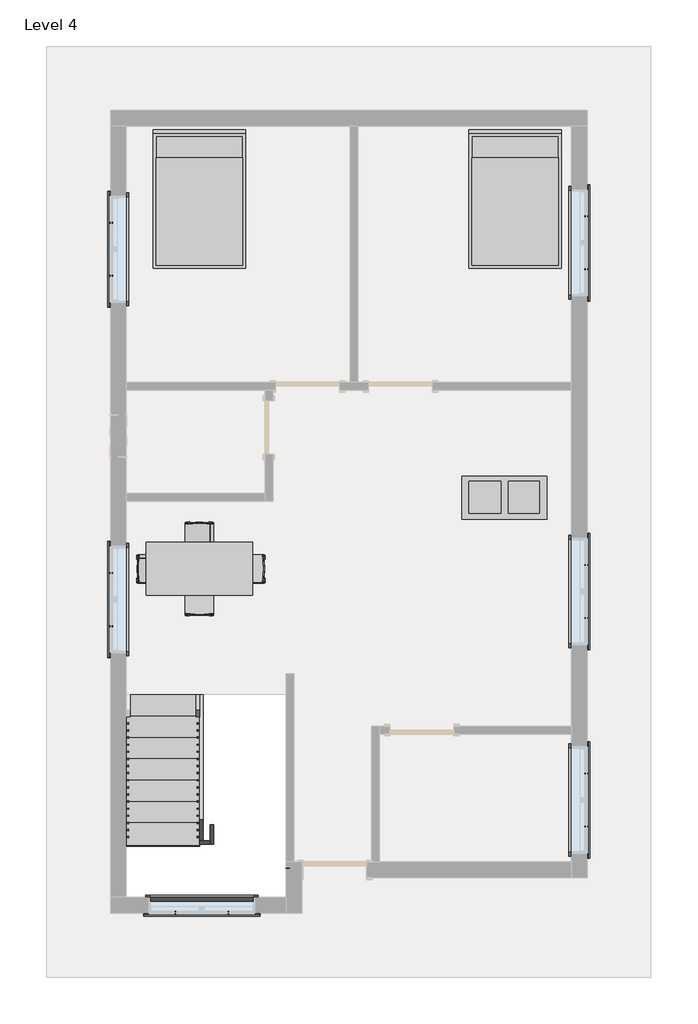
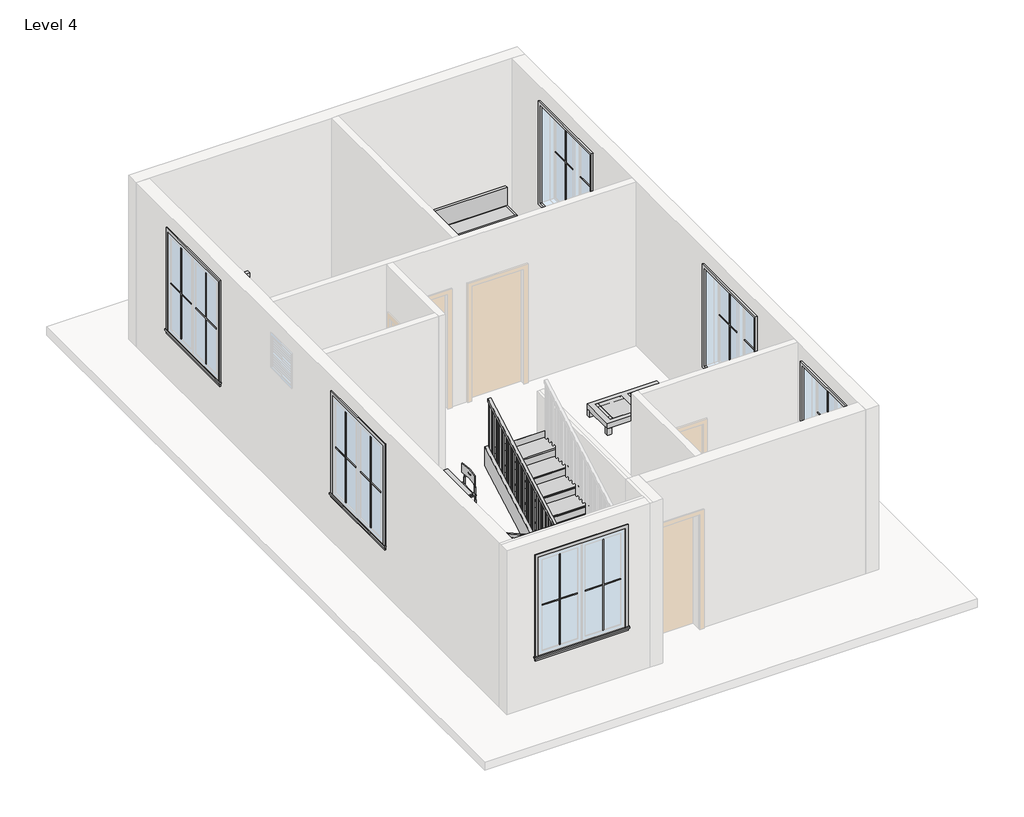
# One storey, part 3 of 3: 25 proxies, 6 members, 3 furniture elements, 1 railing, 1 stair flight.
"""IFC4 building model written with IfcOpenShell, lengths in millimetres."""

from ifc_helpers import new_model, si_unit, frame, origin, place, context, project, spatial, polyline, outline, extrude, faceted_brep, transform, mapped, element, save
from components import muntin_pattern_2x2_muntin_pattern_2x2_f6a80940, muntin_pattern_2x2_muntin_pattern_2x2_09b00a1c, trim_window_exterior_flat_with_sill_698ed857, trim_window_interior_flat_picture_frame_92551a5e, coffee_table_with_brass_mullions_11320_coffee_table_with_5962bef7, bed_17739_bed_17739_15c61121, dining_table_w_chairs_11374_0cdfc61b, stair_flight_f9143c42

model = new_model("IFC4")

# Units and contexts
model_context = context("Model", 3, world=origin())
ifc_project = project(units=[si_unit("LENGTHUNIT", "METRE", prefix="MILLI")], contexts=[model_context])

# Site, building, storey
site = spatial("IfcSite", under=ifc_project)
building = spatial("IfcBuilding", under=site)
storey = spatial("IfcBuildingStorey", under=building, Name="Level 4", Elevation=9448.8)

# Proxies
placement = place(None, origin())
muntin_pattern_2x2_muntin_pattern_2x2_shape = muntin_pattern_2x2_muntin_pattern_2x2_f6a80940(model_context)
element("IfcBuildingElementProxy", 1, Name="Muntin Pattern_2x2 : Muntin Pattern_2x2", ObjectType="Muntin Pattern_2x2 : Muntin Pattern_2x2", at=placement, inside=storey, context=model_context, shape_type="MappedRepresentation", body=[
    mapped(muntin_pattern_2x2_muntin_pattern_2x2_shape, transform((-2773.368364, -6686.2830018, 10433.05), x_axis=(-1.0, 0.0, 0.0), y_axis=(0.0, -1.0, 0.0), z_axis=(0.0, 0.0, 1.0))),
])
element("IfcBuildingElementProxy", 2, Name="Muntin Pattern_2x2 : Muntin Pattern_2x2", ObjectType="Muntin Pattern_2x2 : Muntin Pattern_2x2", at=placement, inside=storey, context=model_context, shape_type="MappedRepresentation", body=[
    mapped(muntin_pattern_2x2_muntin_pattern_2x2_shape, transform((2349.494136, -4693.9705018, 10433.05), x_axis=(0.0, -1.0, 0.0), y_axis=(1.0, 0.0, 0.0), z_axis=(0.0, 0.0, 1.0))),
])
element("IfcBuildingElementProxy", 3, Name="Muntin Pattern_2x2 : Muntin Pattern_2x2", ObjectType="Muntin Pattern_2x2 : Muntin Pattern_2x2", at=placement, inside=storey, context=model_context, shape_type="MappedRepresentation", body=[
    mapped(muntin_pattern_2x2_muntin_pattern_2x2_shape, transform((2349.494136, -1712.6455018, 10433.05), x_axis=(0.0, -1.0, 0.0), y_axis=(1.0, 0.0, 0.0), z_axis=(0.0, 0.0, 1.0))),
])
element("IfcBuildingElementProxy", 4, Name="Muntin Pattern_2x2 : Muntin Pattern_2x2", ObjectType="Muntin Pattern_2x2 : Muntin Pattern_2x2", at=placement, inside=storey, context=model_context, shape_type="MappedRepresentation", body=[
    mapped(muntin_pattern_2x2_muntin_pattern_2x2_shape, transform((-4451.355864, -2586.5525081, 10433.05), x_axis=(0.0, 1.0, 0.0), y_axis=(-1.0, 0.0, 0.0), z_axis=(0.0, 0.0, 1.0))),
])
element("IfcBuildingElementProxy", 5, Name="Muntin Pattern_2x2 : Muntin Pattern_2x2", ObjectType="Muntin Pattern_2x2 : Muntin Pattern_2x2", at=placement, inside=storey, context=model_context, shape_type="MappedRepresentation", body=[
    mapped(muntin_pattern_2x2_muntin_pattern_2x2_shape, transform((2349.494136, 3272.1044982, 10433.05), x_axis=(0.0, -1.0, 0.0), y_axis=(1.0, 0.0, 0.0), z_axis=(0.0, 0.0, 1.0))),
])
element("IfcBuildingElementProxy", 6, Name="Muntin Pattern_2x2 : Muntin Pattern_2x2", ObjectType="Muntin Pattern_2x2 : Muntin Pattern_2x2", at=placement, inside=storey, context=model_context, shape_type="MappedRepresentation", body=[
    mapped(muntin_pattern_2x2_muntin_pattern_2x2_shape, transform((-4451.355864, 2421.2162133, 10433.05), x_axis=(0.0, 1.0, 0.0), y_axis=(-1.0, 0.0, 0.0), z_axis=(0.0, 0.0, 1.0))),
])
muntin_pattern_2x2_muntin_pattern_2x2_2_shape = muntin_pattern_2x2_muntin_pattern_2x2_09b00a1c(model_context)
element("IfcBuildingElementProxy", 7, Name="Muntin Pattern_2x2 : Muntin Pattern_2x2", ObjectType="Muntin Pattern_2x2 : Muntin Pattern_2x2", at=placement, inside=storey, context=model_context, shape_type="MappedRepresentation", body=[
    mapped(muntin_pattern_2x2_muntin_pattern_2x2_2_shape, transform((-3532.193364, -6686.2830018, 10433.05), x_axis=(1.0, 0.0, 0.0), y_axis=(0.0, 1.0, 0.0), z_axis=(0.0, 0.0, 1.0))),
])
element("IfcBuildingElementProxy", 8, Name="Muntin Pattern_2x2 : Muntin Pattern_2x2", ObjectType="Muntin Pattern_2x2 : Muntin Pattern_2x2", at=placement, inside=storey, context=model_context, shape_type="MappedRepresentation", body=[
    mapped(muntin_pattern_2x2_muntin_pattern_2x2_2_shape, transform((2349.494136, -5452.7955018, 10433.05), x_axis=(0.0, 1.0, 0.0), y_axis=(-1.0, 0.0, 0.0), z_axis=(0.0, 0.0, 1.0))),
])
element("IfcBuildingElementProxy", 9, Name="Muntin Pattern_2x2 : Muntin Pattern_2x2", ObjectType="Muntin Pattern_2x2 : Muntin Pattern_2x2", at=placement, inside=storey, context=model_context, shape_type="MappedRepresentation", body=[
    mapped(muntin_pattern_2x2_muntin_pattern_2x2_2_shape, transform((2349.494136, -2471.4705018, 10433.05), x_axis=(0.0, 1.0, 0.0), y_axis=(-1.0, 0.0, 0.0), z_axis=(0.0, 0.0, 1.0))),
])
element("IfcBuildingElementProxy", 10, Name="Muntin Pattern_2x2 : Muntin Pattern_2x2", ObjectType="Muntin Pattern_2x2 : Muntin Pattern_2x2", at=placement, inside=storey, context=model_context, shape_type="MappedRepresentation", body=[
    mapped(muntin_pattern_2x2_muntin_pattern_2x2_2_shape, transform((-4451.355864, -1827.7275081, 10433.05), x_axis=(0.0, -1.0, 0.0), y_axis=(1.0, 0.0, 0.0), z_axis=(0.0, 0.0, 1.0))),
])
element("IfcBuildingElementProxy", 11, Name="Muntin Pattern_2x2 : Muntin Pattern_2x2", ObjectType="Muntin Pattern_2x2 : Muntin Pattern_2x2", at=placement, inside=storey, context=model_context, shape_type="MappedRepresentation", body=[
    mapped(muntin_pattern_2x2_muntin_pattern_2x2_2_shape, transform((2349.494136, 2513.2794982, 10433.05), x_axis=(0.0, 1.0, 0.0), y_axis=(-1.0, 0.0, 0.0), z_axis=(0.0, 0.0, 1.0))),
])
element("IfcBuildingElementProxy", 12, Name="Muntin Pattern_2x2 : Muntin Pattern_2x2", ObjectType="Muntin Pattern_2x2 : Muntin Pattern_2x2", at=placement, inside=storey, context=model_context, shape_type="MappedRepresentation", body=[
    mapped(muntin_pattern_2x2_muntin_pattern_2x2_2_shape, transform((-4451.355864, 3180.0412133, 10433.05), x_axis=(0.0, -1.0, 0.0), y_axis=(1.0, 0.0, 0.0), z_axis=(0.0, 0.0, 1.0))),
])
trim_window_exterior_flat_with_sill_shape = trim_window_exterior_flat_with_sill_698ed857(model_context)
element("IfcBuildingElementProxy", 13, Name="Trim-Window-Exterior-Flat : with Sill", ObjectType="Trim-Window-Exterior-Flat : with Sill", at=placement, inside=storey, context=model_context, shape_type="MappedRepresentation", body=[
    mapped(trim_window_exterior_flat_with_sill_shape, transform((-3152.780864, -6695.8080018, 12192.0), x_axis=(1.0, 0.0, 0.0), y_axis=(0.0, 0.0, 1.0), z_axis=(0.0, -1.0, 0.0))),
])
element("IfcBuildingElementProxy", 14, Name="Trim-Window-Exterior-Flat : with Sill", ObjectType="Trim-Window-Exterior-Flat : with Sill", at=placement, inside=storey, context=model_context, shape_type="MappedRepresentation", body=[
    mapped(trim_window_exterior_flat_with_sill_shape, transform((2359.019136, -5073.3830018, 12192.0), x_axis=(0.0, 1.0, 0.0), y_axis=(0.0, 0.0, 1.0), z_axis=(1.0, 0.0, 0.0))),
])
element("IfcBuildingElementProxy", 15, Name="Trim-Window-Exterior-Flat : with Sill", ObjectType="Trim-Window-Exterior-Flat : with Sill", at=placement, inside=storey, context=model_context, shape_type="MappedRepresentation", body=[
    mapped(trim_window_exterior_flat_with_sill_shape, transform((2359.019136, -2092.0580018, 12192.0), x_axis=(0.0, 1.0, 0.0), y_axis=(0.0, 0.0, 1.0), z_axis=(1.0, 0.0, 0.0))),
])
element("IfcBuildingElementProxy", 16, Name="Trim-Window-Exterior-Flat : with Sill", ObjectType="Trim-Window-Exterior-Flat : with Sill", at=placement, inside=storey, context=model_context, shape_type="MappedRepresentation", body=[
    mapped(trim_window_exterior_flat_with_sill_shape, transform((-4460.880864, -2207.1400081, 12192.0), x_axis=(0.0, -1.0, 0.0), y_axis=(0.0, 0.0, 1.0), z_axis=(-1.0, 0.0, 0.0))),
])
element("IfcBuildingElementProxy", 17, Name="Trim-Window-Exterior-Flat : with Sill", ObjectType="Trim-Window-Exterior-Flat : with Sill", at=placement, inside=storey, context=model_context, shape_type="MappedRepresentation", body=[
    mapped(trim_window_exterior_flat_with_sill_shape, transform((2359.019136, 2892.6919982, 12192.0), x_axis=(0.0, 1.0, 0.0), y_axis=(0.0, 0.0, 1.0), z_axis=(1.0, 0.0, 0.0))),
])
element("IfcBuildingElementProxy", 18, Name="Trim-Window-Exterior-Flat : with Sill", ObjectType="Trim-Window-Exterior-Flat : with Sill", at=placement, inside=storey, context=model_context, shape_type="MappedRepresentation", body=[
    mapped(trim_window_exterior_flat_with_sill_shape, transform((-4460.880864, 2800.6287133, 12192.0), x_axis=(0.0, -1.0, 0.0), y_axis=(0.0, 0.0, 1.0), z_axis=(-1.0, 0.0, 0.0))),
])
trim_window_interior_flat_picture_frame_shape = trim_window_interior_flat_picture_frame_92551a5e(model_context)
element("IfcBuildingElementProxy", 19, Name="Trim-Window-Interior-Flat : Picture Frame", ObjectType="Trim-Window-Interior-Flat : Picture Frame", at=placement, inside=storey, context=model_context, shape_type="MappedRepresentation", body=[
    mapped(trim_window_interior_flat_picture_frame_shape, transform((-3152.780864, -6467.2080018, 12192.0), x_axis=(-1.0, 0.0, 0.0), y_axis=(0.0, 0.0, 1.0), z_axis=(0.0, 1.0, 0.0))),
])
element("IfcBuildingElementProxy", 20, Name="Trim-Window-Interior-Flat : Picture Frame", ObjectType="Trim-Window-Interior-Flat : Picture Frame", at=placement, inside=storey, context=model_context, shape_type="MappedRepresentation", body=[
    mapped(trim_window_interior_flat_picture_frame_shape, transform((2130.419136, -5073.3830018, 12192.0), x_axis=(0.0, -1.0, 0.0), y_axis=(0.0, 0.0, 1.0), z_axis=(-1.0, 0.0, 0.0))),
])
element("IfcBuildingElementProxy", 21, Name="Trim-Window-Interior-Flat : Picture Frame", ObjectType="Trim-Window-Interior-Flat : Picture Frame", at=placement, inside=storey, context=model_context, shape_type="MappedRepresentation", body=[
    mapped(trim_window_interior_flat_picture_frame_shape, transform((2130.419136, -2092.0580018, 12192.0), x_axis=(0.0, -1.0, 0.0), y_axis=(0.0, 0.0, 1.0), z_axis=(-1.0, 0.0, 0.0))),
])
element("IfcBuildingElementProxy", 22, Name="Trim-Window-Interior-Flat : Picture Frame", ObjectType="Trim-Window-Interior-Flat : Picture Frame", at=placement, inside=storey, context=model_context, shape_type="MappedRepresentation", body=[
    mapped(trim_window_interior_flat_picture_frame_shape, transform((-4232.280864, -2207.1400081, 12192.0), x_axis=(0.0, 1.0, 0.0), y_axis=(0.0, 0.0, 1.0), z_axis=(1.0, 0.0, 0.0))),
])
element("IfcBuildingElementProxy", 23, Name="Trim-Window-Interior-Flat : Picture Frame", ObjectType="Trim-Window-Interior-Flat : Picture Frame", at=placement, inside=storey, context=model_context, shape_type="MappedRepresentation", body=[
    mapped(trim_window_interior_flat_picture_frame_shape, transform((2130.419136, 2892.6919982, 12192.0), x_axis=(0.0, -1.0, 0.0), y_axis=(0.0, 0.0, 1.0), z_axis=(-1.0, 0.0, 0.0))),
])
element("IfcBuildingElementProxy", 24, Name="Trim-Window-Interior-Flat : Picture Frame", ObjectType="Trim-Window-Interior-Flat : Picture Frame", at=placement, inside=storey, context=model_context, shape_type="MappedRepresentation", body=[
    mapped(trim_window_interior_flat_picture_frame_shape, transform((-4232.280864, 2800.6287133, 12192.0), x_axis=(0.0, 1.0, 0.0), y_axis=(0.0, 0.0, 1.0), z_axis=(1.0, 0.0, 0.0))),
])
coffee_table_with_brass_mullions_11320_coffee_table_with_shape = coffee_table_with_brass_mullions_11320_coffee_table_with_5962bef7(model_context)
element("IfcBuildingElementProxy", 25, Name="coffee_table_with_brass_mullions_11320 : coffee_table_with_brass_mullions_11320", ObjectType="coffee_table_with_brass_mullions_11320 : coffee_table_with_brass_mullions_11320", at=placement, inside=storey, context=model_context, shape_type="MappedRepresentation", body=[
    mapped(coffee_table_with_brass_mullions_11320_coffee_table_with_shape, transform((1812.3816081, -1181.1001099, 9448.8), x_axis=(1.0, 0.0, 0.0), y_axis=(0.0, 1.0, 0.0), z_axis=(0.0, 0.0, 1.0))),
])

# Furniture
bed_17739_bed_17739_shape = bed_17739_bed_17739_15c61121(model_context)
element("IfcFurniture", 26, ObjectType="Bed_17739 : Bed_17739", at=placement, inside=storey, context=model_context, shape_type="MappedRepresentation", body=[
    mapped(bed_17739_bed_17739_shape, transform((1328.5116081, 3496.3098901, 9448.8), x_axis=(1.0, 0.0, 0.0), y_axis=(0.0, 1.0, 0.0), z_axis=(0.0, 0.0, 1.0))),
])
element("IfcFurniture", 27, ObjectType="Bed_17739 : Bed_17739", at=placement, inside=storey, context=model_context, shape_type="MappedRepresentation", body=[
    mapped(bed_17739_bed_17739_shape, transform((-3187.6083919, 3496.3098901, 9448.8), x_axis=(1.0, 0.0, 0.0), y_axis=(0.0, 1.0, 0.0), z_axis=(0.0, 0.0, 1.0))),
])
dining_table_w_chairs_11374_shape = dining_table_w_chairs_11374_0cdfc61b(model_context)
element("IfcFurniture", 28, ObjectType="Dining_Table_w_Chairs_11374", at=placement, inside=storey, context=model_context, shape_type="MappedRepresentation", body=[
    mapped(dining_table_w_chairs_11374_shape, transform((-3205.8741586, -1863.0511877, 9448.8), x_axis=(1.0, 0.0, 0.0), y_axis=(0.0, 1.0, 0.0), z_axis=(0.0, 0.0, 1.0))),
])

# Members
element("IfcMember", 29, ObjectType="Stringer - 2\" Width", at=placement, inside=storey, context=model_context, shape_type="SweptSolid", body=[
    extrude(outline(polyline([(-3571.6080018, 9656.3983948), (-3571.6080018, 9448.8), (-3825.5525046, 9448.8), (-5654.4080018, 10464.8308318), (-5654.4080018, 10813.5095059), (-3571.6080018, 9656.3983948)])), frame((-3187.6083919, 0.0, 0.0), z_axis=(1.0, 0.0, 0.0), x_axis=(0.0, 1.0, 0.0)), (0.0, 0.0, 1.0), 50.8),
])
element("IfcMember", 30, ObjectType="Stringer - 2\" Width", at=placement, inside=storey, context=model_context, shape_type="SweptSolid", body=[
    extrude(outline(polyline([(-3187.6083919, -5705.2080018), (-3187.6083919, -5654.4080018), (-3035.2083919, -5654.4080018), (-3035.2083919, -5705.2080018), (-3187.6083919, -5705.2080018)])), frame((0.0, 0.0, 10574.8666667), z_axis=(0.0, 0.0, 1.0), x_axis=(1.0, 0.0, 0.0)), (0.0, 0.0, 1.0), 304.8),
])
element("IfcMember", 31, ObjectType="Stringer - 2\" Width", at=placement, inside=storey, context=model_context, shape_type="SweptSolid", body=[
    extrude(outline(polyline([(-5705.2080018, 10574.8666667), (-5705.2080018, 10841.7317281), (-3571.6080018, 12027.0650614), (-3571.6080018, 11678.3863873), (-5557.943499, 10574.8666667), (-5705.2080018, 10574.8666667)])), frame((-3035.2083919, 0.0, 0.0), z_axis=(1.0, 0.0, 0.0), x_axis=(0.0, 1.0, 0.0)), (0.0, 0.0, 1.0), 50.8),
])
element("IfcMember", 32, ObjectType="Stringer - 2\" Width", at=placement, inside=storey, context=model_context, shape_type="SweptSolid", body=[
    extrude(outline(polyline([(-3571.6080018, 9656.3983948), (-3571.6080018, 9448.8), (-3825.5525046, 9448.8), (-6401.1125046, 10879.6666667), (-5773.4908912, 10879.6666667), (-3571.6080018, 9656.3983948)])), frame((-4283.080864, 0.0, 0.0), z_axis=(1.0, 0.0, 0.0), x_axis=(0.0, 1.0, 0.0)), (0.0, 0.0, 1.0), 50.8),
])
element("IfcMember", 33, ObjectType="Stringer - 2\" Width", at=placement, inside=storey, context=model_context, shape_type="SweptSolid", body=[
    extrude(outline(polyline([(-4283.080864, -6518.0080018), (-4283.080864, -6467.2080018), (-1946.280864, -6467.2080018), (-1946.280864, -6518.0080018), (-4283.080864, -6518.0080018)])), frame((0.0, 0.0, 10574.8666667), z_axis=(0.0, 0.0, 1.0), x_axis=(1.0, 0.0, 0.0)), (0.0, 0.0, 1.0), 304.8),
])
element("IfcMember", 34, ObjectType="Stringer - 2\" Width", at=placement, inside=storey, context=model_context, shape_type="SweptSolid", body=[
    extrude(outline(polyline([(-6185.5651124, 10574.8666667), (-3571.6080018, 12027.0650614), (-3571.6080018, 11678.3863873), (-5557.943499, 10574.8666667), (-6185.5651124, 10574.8666667)])), frame((-1946.280864, 0.0, 0.0), z_axis=(1.0, 0.0, 0.0), x_axis=(0.0, 1.0, 0.0)), (0.0, 0.0, 1.0), 50.8),
])

# Railing
element("IfcRailing", 35, ObjectType="Handrail - Rectangular", at=placement, inside=storey, context=model_context, shape_type="SolidModel", body=[
    faceted_brep([(-3187.6083919, -3571.6080018, 10532.5333333), (-3187.6083919, -3571.6080018, 10474.420221), (-3238.4083919, -3571.6080018, 10474.420221), (-3238.4083919, -3571.6080018, 10532.5333333), (-3187.6083919, -5629.0080018, 11675.5333333), (-3187.6083919, -5679.8080018, 11645.6424432), (-3238.4083919, -5679.8080018, 11645.6424432), (-3238.4083919, -5629.0080018, 11675.5333333), (-3187.6083919, -5629.0080018, 11717.8666667), (-3187.6083919, -5679.8080018, 11667.0666667), (-3238.4083919, -5679.8080018, 11667.0666667), (-3238.4083919, -5629.0080018, 11717.8666667), (-3187.6083919, -5705.2080018, 11717.8666667), (-3187.6083919, -5705.2080018, 11667.0666667), (-3238.4083919, -5756.0080018, 11667.0666667), (-3238.4083919, -5756.0080018, 11717.8666667), (-3111.4083919, -5705.2080018, 11717.8666667), (-3111.4083919, -5705.2080018, 11667.0666667), (-3111.4083919, -5756.0080018, 11667.0666667), (-3111.4083919, -5756.0080018, 11717.8666667), (-3060.6083919, -5705.2080018, 11717.8666667), (-3009.8083919, -5705.2080018, 11667.0666667), (-3009.8083919, -5756.0080018, 11667.0666667), (-3060.6083919, -5756.0080018, 11717.8666667), (-3060.6083919, -5705.2080018, 11760.2), (-3009.8083919, -5705.2080018, 11709.4), (-3009.8083919, -5756.0080018, 11709.4), (-3060.6083919, -5756.0080018, 11760.2), (-2984.4083919, -5705.2080018, 11760.2), (-2984.4083919, -5705.2080018, 11709.4), (-2933.6083919, -5756.0080018, 11709.4), (-2933.6083919, -5756.0080018, 11760.2), (-2984.4083919, -5629.0080018, 11760.2), (-2984.4083919, -5615.8443995, 11709.4), (-2933.6083919, -5615.8443995, 11709.4), (-2933.6083919, -5629.0080018, 11760.2), (-2984.4083919, -3571.6080018, 12903.2), (-2933.6083919, -3571.6080018, 12903.2), (-2933.6083919, -3571.6080018, 12845.0868876), (-2984.4083919, -3571.6080018, 12845.0868876)], [[[0, 1, 2, 3]], [[1, 0, 4, 5]], [[2, 1, 5, 6]], [[3, 2, 6, 7]], [[0, 3, 7, 4]], [[5, 4, 8, 9]], [[6, 5, 9, 10]], [[7, 6, 10, 11]], [[4, 7, 11, 8]], [[9, 8, 12, 13]], [[10, 9, 13, 14]], [[11, 10, 14, 15]], [[8, 11, 15, 12]], [[13, 12, 16, 17]], [[14, 13, 17, 18]], [[15, 14, 18, 19]], [[12, 15, 19, 16]], [[17, 16, 20, 21]], [[18, 17, 21, 22]], [[19, 18, 22, 23]], [[16, 19, 23, 20]], [[21, 20, 24, 25]], [[22, 21, 25, 26]], [[23, 22, 26, 27]], [[20, 23, 27, 24]], [[25, 24, 28, 29]], [[26, 25, 29, 30]], [[27, 26, 30, 31]], [[24, 27, 31, 28]], [[29, 28, 32, 33]], [[30, 29, 33, 34]], [[31, 30, 34, 35]], [[28, 31, 35, 32]], [[36, 37, 38, 39]], [[33, 32, 36, 39]], [[34, 33, 39, 38]], [[35, 34, 38, 37]], [[32, 35, 37, 36]]]),
    extrude(outline(polyline([(-3587.4830018, 12836.2674432), (-3587.4830018, 11819.4666667), (-3606.5330018, 11819.4666667), (-3606.5330018, 12825.6841099), (-3587.4830018, 12836.2674432)])), frame((-2968.5333919, 0.0, 0.0), z_axis=(1.0, 0.0, 0.0), x_axis=(0.0, 1.0, 0.0)), (0.0, 0.0, 1.0), 19.05),
    extrude(outline(polyline([(-3689.0830018, 12779.8229988), (-3689.0830018, 11819.4666667), (-3708.1330018, 11819.4666667), (-3708.1330018, 12769.2396654), (-3689.0830018, 12779.8229988)])), frame((-2968.5333919, 0.0, 0.0), z_axis=(1.0, 0.0, 0.0), x_axis=(0.0, 1.0, 0.0)), (0.0, 0.0, 1.0), 19.05),
    extrude(outline(polyline([(-3790.6830018, 12723.3785543), (-3790.6830018, 11819.4666667), (-3809.7330018, 11819.4666667), (-3809.7330018, 12712.795221), (-3790.6830018, 12723.3785543)])), frame((-2968.5333919, 0.0, 0.0), z_axis=(1.0, 0.0, 0.0), x_axis=(0.0, 1.0, 0.0)), (0.0, 0.0, 1.0), 19.05),
    extrude(outline(polyline([(-3892.2830018, 12666.9341099), (-3892.2830018, 11650.1333333), (-3911.3330018, 11650.1333333), (-3911.3330018, 12656.3507765), (-3892.2830018, 12666.9341099)])), frame((-2968.5333919, 0.0, 0.0), z_axis=(1.0, 0.0, 0.0), x_axis=(0.0, 1.0, 0.0)), (0.0, 0.0, 1.0), 19.05),
    extrude(outline(polyline([(-3993.8830018, 12610.4896654), (-3993.8830018, 11650.1333333), (-4012.9330018, 11650.1333333), (-4012.9330018, 12599.9063321), (-3993.8830018, 12610.4896654)])), frame((-2968.5333919, 0.0, 0.0), z_axis=(1.0, 0.0, 0.0), x_axis=(0.0, 1.0, 0.0)), (0.0, 0.0, 1.0), 19.05),
    extrude(outline(polyline([(-4095.4830018, 12554.045221), (-4095.4830018, 11650.1333333), (-4114.5330018, 11650.1333333), (-4114.5330018, 12543.4618876), (-4095.4830018, 12554.045221)])), frame((-2968.5333919, 0.0, 0.0), z_axis=(1.0, 0.0, 0.0), x_axis=(0.0, 1.0, 0.0)), (0.0, 0.0, 1.0), 19.05),
    extrude(outline(polyline([(-4197.0830018, 12497.6007765), (-4197.0830018, 11480.8), (-4216.1330018, 11480.8), (-4216.1330018, 12487.0174432), (-4197.0830018, 12497.6007765)])), frame((-2968.5333919, 0.0, 0.0), z_axis=(1.0, 0.0, 0.0), x_axis=(0.0, 1.0, 0.0)), (0.0, 0.0, 1.0), 19.05),
    extrude(outline(polyline([(-4298.6830018, 12441.1563321), (-4298.6830018, 11480.8), (-4317.7330018, 11480.8), (-4317.7330018, 12430.5729988), (-4298.6830018, 12441.1563321)])), frame((-2968.5333919, 0.0, 0.0), z_axis=(1.0, 0.0, 0.0), x_axis=(0.0, 1.0, 0.0)), (0.0, 0.0, 1.0), 19.05),
    extrude(outline(polyline([(-4400.2830018, 12384.7118876), (-4400.2830018, 11480.8), (-4419.3330018, 11480.8), (-4419.3330018, 12374.1285543), (-4400.2830018, 12384.7118876)])), frame((-2968.5333919, 0.0, 0.0), z_axis=(1.0, 0.0, 0.0), x_axis=(0.0, 1.0, 0.0)), (0.0, 0.0, 1.0), 19.05),
    extrude(outline(polyline([(-4501.8830018, 12328.2674432), (-4501.8830018, 11311.4666667), (-4520.9330018, 11311.4666667), (-4520.9330018, 12317.6841099), (-4501.8830018, 12328.2674432)])), frame((-2968.5333919, 0.0, 0.0), z_axis=(1.0, 0.0, 0.0), x_axis=(0.0, 1.0, 0.0)), (0.0, 0.0, 1.0), 19.05),
    extrude(outline(polyline([(-4603.4830018, 12271.8229988), (-4603.4830018, 11311.4666667), (-4622.5330018, 11311.4666667), (-4622.5330018, 12261.2396654), (-4603.4830018, 12271.8229988)])), frame((-2968.5333919, 0.0, 0.0), z_axis=(1.0, 0.0, 0.0), x_axis=(0.0, 1.0, 0.0)), (0.0, 0.0, 1.0), 19.05),
    extrude(outline(polyline([(-4705.0830018, 12215.3785543), (-4705.0830018, 11311.4666667), (-4724.1330018, 11311.4666667), (-4724.1330018, 12204.795221), (-4705.0830018, 12215.3785543)])), frame((-2968.5333919, 0.0, 0.0), z_axis=(1.0, 0.0, 0.0), x_axis=(0.0, 1.0, 0.0)), (0.0, 0.0, 1.0), 19.05),
    extrude(outline(polyline([(-4806.6830018, 12158.9341099), (-4806.6830018, 11142.1333333), (-4825.7330018, 11142.1333333), (-4825.7330018, 12148.3507765), (-4806.6830018, 12158.9341099)])), frame((-2968.5333919, 0.0, 0.0), z_axis=(1.0, 0.0, 0.0), x_axis=(0.0, 1.0, 0.0)), (0.0, 0.0, 1.0), 19.05),
    extrude(outline(polyline([(-4908.2830018, 12102.4896654), (-4908.2830018, 11142.1333333), (-4927.3330018, 11142.1333333), (-4927.3330018, 12091.9063321), (-4908.2830018, 12102.4896654)])), frame((-2968.5333919, 0.0, 0.0), z_axis=(1.0, 0.0, 0.0), x_axis=(0.0, 1.0, 0.0)), (0.0, 0.0, 1.0), 19.05),
    extrude(outline(polyline([(-5009.8830018, 12046.045221), (-5009.8830018, 11142.1333333), (-5028.9330018, 11142.1333333), (-5028.9330018, 12035.4618876), (-5009.8830018, 12046.045221)])), frame((-2968.5333919, 0.0, 0.0), z_axis=(1.0, 0.0, 0.0), x_axis=(0.0, 1.0, 0.0)), (0.0, 0.0, 1.0), 19.05),
    extrude(outline(polyline([(-5111.4830018, 11989.6007765), (-5111.4830018, 10972.8), (-5130.5330018, 10972.8), (-5130.5330018, 11979.0174432), (-5111.4830018, 11989.6007765)])), frame((-2968.5333919, 0.0, 0.0), z_axis=(1.0, 0.0, 0.0), x_axis=(0.0, 1.0, 0.0)), (0.0, 0.0, 1.0), 19.05),
    extrude(outline(polyline([(-5213.0830018, 11933.1563321), (-5213.0830018, 10972.8), (-5232.1330018, 10972.8), (-5232.1330018, 11922.5729988), (-5213.0830018, 11933.1563321)])), frame((-2968.5333919, 0.0, 0.0), z_axis=(1.0, 0.0, 0.0), x_axis=(0.0, 1.0, 0.0)), (0.0, 0.0, 1.0), 19.05),
    extrude(outline(polyline([(-5314.6830018, 11876.7118876), (-5314.6830018, 10972.8), (-5333.7330018, 10972.8), (-5333.7330018, 11866.1285543), (-5314.6830018, 11876.7118876)])), frame((-2968.5333919, 0.0, 0.0), z_axis=(1.0, 0.0, 0.0), x_axis=(0.0, 1.0, 0.0)), (0.0, 0.0, 1.0), 19.05),
    extrude(outline(polyline([(-5416.2830018, 11820.2674432), (-5416.2830018, 10803.4666667), (-5435.3330018, 10803.4666667), (-5435.3330018, 11809.6841099), (-5416.2830018, 11820.2674432)])), frame((-2968.5333919, 0.0, 0.0), z_axis=(1.0, 0.0, 0.0), x_axis=(0.0, 1.0, 0.0)), (0.0, 0.0, 1.0), 19.05),
    extrude(outline(polyline([(-5517.8830018, 11763.8229988), (-5517.8830018, 10803.4666667), (-5536.9330018, 10803.4666667), (-5536.9330018, 11753.2396654), (-5517.8830018, 11763.8229988)])), frame((-2968.5333919, 0.0, 0.0), z_axis=(1.0, 0.0, 0.0), x_axis=(0.0, 1.0, 0.0)), (0.0, 0.0, 1.0), 19.05),
    extrude(outline(polyline([(-5619.4830018, 11707.3785543), (-5619.4830018, 10803.4666667), (-5638.5330018, 10803.4666667), (-5638.5330018, 11696.795221), (-5619.4830018, 11707.3785543)])), frame((-2968.5333919, 0.0, 0.0), z_axis=(1.0, 0.0, 0.0), x_axis=(0.0, 1.0, 0.0)), (0.0, 0.0, 1.0), 19.05),
    extrude(outline(polyline([(-3019.3333919, -5721.0830018), (-3000.2833919, -5721.0830018), (-3000.2833919, -5740.1330018), (-3019.3333919, -5740.1330018), (-3019.3333919, -5721.0830018)])), frame((0.0, 0.0, 10803.4666667), z_axis=(0.0, 0.0, 1.0), x_axis=(1.0, 0.0, 0.0)), (0.0, 0.0, 1.0), 905.9333333),
    extrude(outline(polyline([(-3120.9333919, -5721.0830018), (-3101.8833919, -5721.0830018), (-3101.8833919, -5740.1330018), (-3120.9333919, -5740.1330018), (-3120.9333919, -5721.0830018)])), frame((0.0, 0.0, 10803.4666667), z_axis=(0.0, 0.0, 1.0), x_axis=(1.0, 0.0, 0.0)), (0.0, 0.0, 1.0), 863.6),
    extrude(outline(polyline([(-3203.4833919, -5695.6830018), (-3203.4833919, -5714.7330018), (-3222.5333919, -5714.7330018), (-3222.5333919, -5695.6830018), (-3203.4833919, -5695.6830018)])), frame((0.0, 0.0, 10803.4666667), z_axis=(0.0, 0.0, 1.0), x_axis=(1.0, 0.0, 0.0)), (0.0, 0.0, 1.0), 863.6),
    extrude(outline(polyline([(-5594.0830018, 11598.0174432), (-5594.0830018, 10634.1333333), (-5613.1330018, 10634.1333333), (-5613.1330018, 11608.6007765), (-5594.0830018, 11598.0174432)])), frame((-3222.5333919, 0.0, 0.0), z_axis=(1.0, 0.0, 0.0), x_axis=(0.0, 1.0, 0.0)), (0.0, 0.0, 1.0), 19.05),
    extrude(outline(polyline([(-5492.4830018, 11541.5729988), (-5492.4830018, 10634.1333333), (-5511.5330018, 10634.1333333), (-5511.5330018, 11552.1563321), (-5492.4830018, 11541.5729988)])), frame((-3222.5333919, 0.0, 0.0), z_axis=(1.0, 0.0, 0.0), x_axis=(0.0, 1.0, 0.0)), (0.0, 0.0, 1.0), 19.05),
    extrude(outline(polyline([(-5390.8830018, 11485.1285543), (-5390.8830018, 10634.1333333), (-5409.9330018, 10634.1333333), (-5409.9330018, 11495.7118876), (-5390.8830018, 11485.1285543)])), frame((-3222.5333919, 0.0, 0.0), z_axis=(1.0, 0.0, 0.0), x_axis=(0.0, 1.0, 0.0)), (0.0, 0.0, 1.0), 19.05),
    extrude(outline(polyline([(-5289.2830018, 11428.6841099), (-5289.2830018, 10464.8), (-5308.3330018, 10464.8), (-5308.3330018, 11439.2674432), (-5289.2830018, 11428.6841099)])), frame((-3222.5333919, 0.0, 0.0), z_axis=(1.0, 0.0, 0.0), x_axis=(0.0, 1.0, 0.0)), (0.0, 0.0, 1.0), 19.05),
    extrude(outline(polyline([(-5187.6830018, 11372.2396654), (-5187.6830018, 10464.8), (-5206.7330018, 10464.8), (-5206.7330018, 11382.8229988), (-5187.6830018, 11372.2396654)])), frame((-3222.5333919, 0.0, 0.0), z_axis=(1.0, 0.0, 0.0), x_axis=(0.0, 1.0, 0.0)), (0.0, 0.0, 1.0), 19.05),
    extrude(outline(polyline([(-5086.0830018, 11315.795221), (-5086.0830018, 10464.8), (-5105.1330018, 10464.8), (-5105.1330018, 11326.3785543), (-5086.0830018, 11315.795221)])), frame((-3222.5333919, 0.0, 0.0), z_axis=(1.0, 0.0, 0.0), x_axis=(0.0, 1.0, 0.0)), (0.0, 0.0, 1.0), 19.05),
    extrude(outline(polyline([(-4984.4830018, 11259.3507765), (-4984.4830018, 10295.4666667), (-5003.5330018, 10295.4666667), (-5003.5330018, 11269.9341099), (-4984.4830018, 11259.3507765)])), frame((-3222.5333919, 0.0, 0.0), z_axis=(1.0, 0.0, 0.0), x_axis=(0.0, 1.0, 0.0)), (0.0, 0.0, 1.0), 19.05),
    extrude(outline(polyline([(-4882.8830018, 11202.9063321), (-4882.8830018, 10295.4666667), (-4901.9330018, 10295.4666667), (-4901.9330018, 11213.4896654), (-4882.8830018, 11202.9063321)])), frame((-3222.5333919, 0.0, 0.0), z_axis=(1.0, 0.0, 0.0), x_axis=(0.0, 1.0, 0.0)), (0.0, 0.0, 1.0), 19.05),
    extrude(outline(polyline([(-4781.2830018, 11146.4618876), (-4781.2830018, 10295.4666667), (-4800.3330018, 10295.4666667), (-4800.3330018, 11157.045221), (-4781.2830018, 11146.4618876)])), frame((-3222.5333919, 0.0, 0.0), z_axis=(1.0, 0.0, 0.0), x_axis=(0.0, 1.0, 0.0)), (0.0, 0.0, 1.0), 19.05),
    extrude(outline(polyline([(-4679.6830018, 11090.0174432), (-4679.6830018, 10126.1333333), (-4698.7330018, 10126.1333333), (-4698.7330018, 11100.6007765), (-4679.6830018, 11090.0174432)])), frame((-3222.5333919, 0.0, 0.0), z_axis=(1.0, 0.0, 0.0), x_axis=(0.0, 1.0, 0.0)), (0.0, 0.0, 1.0), 19.05),
    extrude(outline(polyline([(-4578.0830018, 11033.5729988), (-4578.0830018, 10126.1333333), (-4597.1330018, 10126.1333333), (-4597.1330018, 11044.1563321), (-4578.0830018, 11033.5729988)])), frame((-3222.5333919, 0.0, 0.0), z_axis=(1.0, 0.0, 0.0), x_axis=(0.0, 1.0, 0.0)), (0.0, 0.0, 1.0), 19.05),
    extrude(outline(polyline([(-4476.4830018, 10977.1285543), (-4476.4830018, 10126.1333333), (-4495.5330018, 10126.1333333), (-4495.5330018, 10987.7118876), (-4476.4830018, 10977.1285543)])), frame((-3222.5333919, 0.0, 0.0), z_axis=(1.0, 0.0, 0.0), x_axis=(0.0, 1.0, 0.0)), (0.0, 0.0, 1.0), 19.05),
    extrude(outline(polyline([(-4374.8830018, 10920.6841099), (-4374.8830018, 9956.8), (-4393.9330018, 9956.8), (-4393.9330018, 10931.2674432), (-4374.8830018, 10920.6841099)])), frame((-3222.5333919, 0.0, 0.0), z_axis=(1.0, 0.0, 0.0), x_axis=(0.0, 1.0, 0.0)), (0.0, 0.0, 1.0), 19.05),
    extrude(outline(polyline([(-4273.2830018, 10864.2396654), (-4273.2830018, 9956.8), (-4292.3330018, 9956.8), (-4292.3330018, 10874.8229988), (-4273.2830018, 10864.2396654)])), frame((-3222.5333919, 0.0, 0.0), z_axis=(1.0, 0.0, 0.0), x_axis=(0.0, 1.0, 0.0)), (0.0, 0.0, 1.0), 19.05),
    extrude(outline(polyline([(-4171.6830018, 10807.795221), (-4171.6830018, 9956.8), (-4190.7330018, 9956.8), (-4190.7330018, 10818.3785543), (-4171.6830018, 10807.795221)])), frame((-3222.5333919, 0.0, 0.0), z_axis=(1.0, 0.0, 0.0), x_axis=(0.0, 1.0, 0.0)), (0.0, 0.0, 1.0), 19.05),
    extrude(outline(polyline([(-4070.0830018, 10751.3507765), (-4070.0830018, 9787.4666667), (-4089.1330018, 9787.4666667), (-4089.1330018, 10761.9341099), (-4070.0830018, 10751.3507765)])), frame((-3222.5333919, 0.0, 0.0), z_axis=(1.0, 0.0, 0.0), x_axis=(0.0, 1.0, 0.0)), (0.0, 0.0, 1.0), 19.05),
    extrude(outline(polyline([(-3968.4830018, 10694.9063321), (-3968.4830018, 9787.4666667), (-3987.5330018, 9787.4666667), (-3987.5330018, 10705.4896654), (-3968.4830018, 10694.9063321)])), frame((-3222.5333919, 0.0, 0.0), z_axis=(1.0, 0.0, 0.0), x_axis=(0.0, 1.0, 0.0)), (0.0, 0.0, 1.0), 19.05),
    extrude(outline(polyline([(-3866.8830018, 10638.4618876), (-3866.8830018, 9787.4666667), (-3885.9330018, 9787.4666667), (-3885.9330018, 10649.045221), (-3866.8830018, 10638.4618876)])), frame((-3222.5333919, 0.0, 0.0), z_axis=(1.0, 0.0, 0.0), x_axis=(0.0, 1.0, 0.0)), (0.0, 0.0, 1.0), 19.05),
    extrude(outline(polyline([(-3765.2830018, 10582.0174432), (-3765.2830018, 9618.1333333), (-3784.3330018, 9618.1333333), (-3784.3330018, 10592.6007765), (-3765.2830018, 10582.0174432)])), frame((-3222.5333919, 0.0, 0.0), z_axis=(1.0, 0.0, 0.0), x_axis=(0.0, 1.0, 0.0)), (0.0, 0.0, 1.0), 19.05),
    extrude(outline(polyline([(-3663.6830018, 10525.5729988), (-3663.6830018, 9618.1333333), (-3682.7330018, 9618.1333333), (-3682.7330018, 10536.1563321), (-3663.6830018, 10525.5729988)])), frame((-3222.5333919, 0.0, 0.0), z_axis=(1.0, 0.0, 0.0), x_axis=(0.0, 1.0, 0.0)), (0.0, 0.0, 1.0), 19.05),
    extrude(outline(polyline([(-2968.5333919, -5721.0830018), (-2949.4833919, -5721.0830018), (-2949.4833919, -5740.1330018), (-2968.5333919, -5740.1330018), (-2968.5333919, -5721.0830018)])), frame((0.0, 0.0, 10803.4666667), z_axis=(0.0, 0.0, 1.0), x_axis=(1.0, 0.0, 0.0)), (0.0, 0.0, 1.0), 905.9333333),
    extrude(outline(polyline([(-3203.4833919, -5721.0830018), (-3203.4833919, -5740.1330018), (-3222.5333919, -5740.1330018), (-3222.5333919, -5721.0830018), (-3203.4833919, -5721.0830018)])), frame((0.0, 0.0, 10803.4666667), z_axis=(0.0, 0.0, 1.0), x_axis=(1.0, 0.0, 0.0)), (0.0, 0.0, 1.0), 863.6),
    extrude(outline(polyline([(-3571.6080018, 12845.0868876), (-3571.6080018, 11819.4666667), (-3590.6580018, 11819.4666667), (-3590.6580018, 12834.5035543), (-3571.6080018, 12845.0868876)])), frame((-2968.5333919, 0.0, 0.0), z_axis=(1.0, 0.0, 0.0), x_axis=(0.0, 1.0, 0.0)), (0.0, 0.0, 1.0), 19.05),
    extrude(outline(polyline([(-3571.6080018, 10474.420221), (-3571.6080018, 9618.1333333), (-3590.6580018, 9618.1333333), (-3590.6580018, 10485.0035543), (-3571.6080018, 10474.420221)])), frame((-3222.5333919, 0.0, 0.0), z_axis=(1.0, 0.0, 0.0), x_axis=(0.0, 1.0, 0.0)), (0.0, 0.0, 1.0), 19.05),
])

# Stair flight
stair_flight_shape = stair_flight_f9143c42(model_context)
element("IfcStairFlight", 36, ObjectType="2\" Tread 1\" Nosing 1/4\" Riser", at=placement, inside=storey, context=model_context, shape_type="MappedRepresentation", body=[
    mapped(stair_flight_shape, transform((0.0, 0.0, 0.0), x_axis=(1.0, 0.0, 0.0), y_axis=(0.0, 1.0, 0.0), z_axis=(0.0, 0.0, 1.0))),
])

save(model, "model.ifc")

# Revit data of these elements
# Type "Muntin Pattern_2x2 : Muntin Pattern_2x2"
#   Width [instance default] = 4' - 0"
#   Thickness = 0' - 0 1/2"
#   Height [instance default] = 4' - 0"
#   Distance = 0' - 0 3/4"
#   Interior Material [instance default] = none
#   Exterior Material [instance default] = none
#   Default Elevation = 0
# Type "Trim-Window-Exterior-Flat : with Sill"
#   Trim Width = 0' - 2 1/4"
#   Trim Thickness_Picture Frame = 0' - 1 1/4"
#   Trim Thickness_with Sill = 0' - 0 3/4"
#   Sill Thickness = 0' - 1 1/4"
#   Opening Width [instance default] = 2' - 0"
#   Opening Height [instance default] = 3' - 0"
#   Default Elevation = 4' - 0"
#   Sill = yes
#   Picture Frame = no
#   Trim Material [instance default] = none
# Type "Trim-Window-Interior-Flat : Picture Frame"
#   Trim Thickness_Picture Frame = 0' - 1 1/4"
#   Trim Width = 0' - 2 1/4"
#   Trim Thickness_with Sill = 0' - 0 3/4"
#   Sill Thickness = 0' - 1 1/4"
#   Opening Width [instance default] = 2' - 0"
#   Opening Height [instance default] = 3' - 0"
#   Default Elevation = 4' - 0"
#   Sill = no
#   Picture Frame = yes
#   Trim Material [instance default] = none
# Type "coffee_table_with_brass_mullions_11320 : coffee_table_with_brass_mullions_11320"
#   Default Elevation = 0
# Type "Bed_17739 : Bed_17739"
#   Default Elevation = 0
# Type "Dining_Table_w_Chairs_11374"
#   Default Elevation = 0
#   Assembly Code = ""
# Type "Handrail - Rectangular"
#   Assembly Code = "C2010400"
#   built-in parameter 1008612 = 0.0416667 (stored number, unit not read)
#   built-in parameter 1008611 = 0.0416667 (stored number, unit not read)
#   built-in parameter 1008609 = 0.333333 (stored number, unit not read)
#   built-in parameter 1008604 = 0.166667 (stored number, unit not read)
#   built-in parameter 1008603 = 0.166667 (stored number, unit not read)
#   Railing Height = 3' - 0"
#   built-in parameter 1008630 = 2
#   built-in parameter 1008610 = 2
#   built-in parameter 1008618 = Baluster - Square : 3/4"
# Elements 1, 2, 3, 4, 5, 6, 7, 8, 9, 10, 11, 12 (IfcBuildingElementProxy, "Muntin Pattern_2x2 : Muntin Pattern_2x2")
#   Width = 2' - 0 5/8"
#   Height = 5' - 6 1/2"
#   Interior Material = Wood - Stained
#   Exterior Material = Clad - White
#   Phase Created = New Construction
#   Materials on its faces: "Clad - White", "Wood - Stained"
# Elements 13, 14, 15, 16, 17, 18 (IfcBuildingElementProxy, "Trim-Window-Exterior-Flat : with Sill")
#   Opening Width = 5' - 0"
#   Opening Height = 6' - 0"
#   Trim Material = Clad - White
#   Phase Created = New Construction
#   Materials on its faces: "Clad - White"
# Elements 19, 20, 21, 22, 23, 24 (IfcBuildingElementProxy, "Trim-Window-Interior-Flat : Picture Frame")
#   Opening Width = 5' - 0"
#   Opening Height = 6' - 0"
#   Trim Material = Wood - Stained
#   Phase Created = New Construction
#   Materials on its faces: "Wood - Stained"
# Element 25 (IfcBuildingElementProxy, "coffee_table_with_brass_mullions_11320 : coffee_table_with_brass_mullions_11320")
#   Phase Created = New Construction
#   Materials on its faces: "Default Wall", "TABLE", "Glass", "Default"
# Elements 26, 27 (IfcFurniture, "Bed_17739 : Bed_17739")
#   Phase Created = New Construction
#   Materials on its faces: "legs", "sheets", "bed frame", "Blanket"
# Element 28 (IfcFurniture, "Dining_Table_w_Chairs_11374")
#   Phase Created = New Construction
# Elements 29, 30, 31, 32, 33, 34 (IfcMember, "Stringer - 2\" Width")
#   Phase Created = New Construction
# Element 35 (IfcRailing, "Handrail - Rectangular")
#   Phase Created = New Construction
# Element 36 (IfcStairFlight, "2\" Tread 1\" Nosing 1/4\" Riser")
#   Phase Created = New Construction
# Materials
#   "Clad - White": class "Wood", colour RGB 242 242 238, transparency 0, Cost = 0
#   "Wood - Stained": class "Wood", colour RGB 224 178 126, transparency 0, Cost = 0
#   "Default Wall": colour RGB 128 128 128, transparency 0, Cost = 0
#   "TABLE": class "Generic", colour RGB 120 120 120, transparency 0, Cost = 0
#   "Glass": class "Glass", colour RGB 0 128 192, transparency 0.75, Description = "Soda Lime Glass", Cost = 0
#   "Default": colour RGB 127 127 127, transparency 0, Cost = 0
#   "legs": colour RGB 90 73 37, transparency 0, Cost = 0
#   "sheets": colour RGB 200 195 176, transparency 0, Cost = 0
#   "bed frame": colour RGB 90 73 37, transparency 0, Cost = 0
#   "Blanket": class "System", colour RGB 59 0 1, transparency 0, Cost = 0
